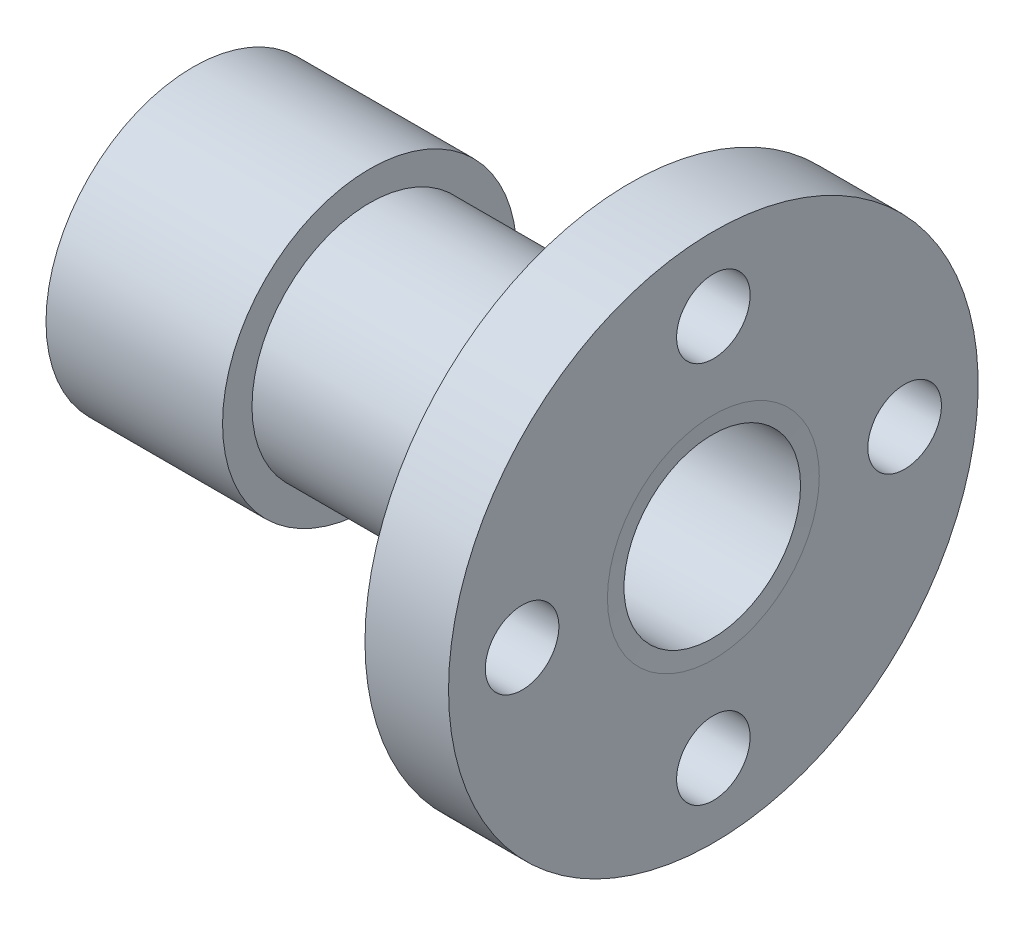
ISO-10303-21;
HEADER;
FILE_DESCRIPTION(('STEP AP214'),'2;1');
FILE_NAME('part.step','',(''),(''),'','','');
FILE_SCHEMA(('AUTOMOTIVE_DESIGN { 1 0 10303 214 1 1 1 1 }'));
ENDSEC;
DATA;
#1=APPLICATION_CONTEXT('core data for automotive mechanical design processes');
#2=APPLICATION_PROTOCOL_DEFINITION('international standard','automotive_design',2000,#1);
#3=PRODUCT_CONTEXT('',#1,'mechanical');
#4=PRODUCT('Part','Part','',(#3));
#5=PRODUCT_RELATED_PRODUCT_CATEGORY('part','',(#4));
#6=PRODUCT_DEFINITION_FORMATION('','',#4);
#7=PRODUCT_DEFINITION_CONTEXT('part definition',#1,'design');
#8=PRODUCT_DEFINITION('design','',#6,#7);
#9=PRODUCT_DEFINITION_SHAPE('','',#8);
#10=(LENGTH_UNIT() NAMED_UNIT(*) SI_UNIT(.MILLI.,.METRE.));
#11=(NAMED_UNIT(*) PLANE_ANGLE_UNIT() SI_UNIT($,.RADIAN.));
#12=(NAMED_UNIT(*) SI_UNIT($,.STERADIAN.) SOLID_ANGLE_UNIT());
#13=UNCERTAINTY_MEASURE_WITH_UNIT(LENGTH_MEASURE(1.E-05),#10,'distance_accuracy_value','');
#14=(GEOMETRIC_REPRESENTATION_CONTEXT(3) GLOBAL_UNCERTAINTY_ASSIGNED_CONTEXT((#13)) GLOBAL_UNIT_ASSIGNED_CONTEXT((#10,
#11,#12)) REPRESENTATION_CONTEXT('',''));
#15=CARTESIAN_POINT('',(0.,0.,0.));
#16=DIRECTION('',(0.,0.,1.));
#17=DIRECTION('',(1.,0.,0.));
#18=AXIS2_PLACEMENT_3D('',#15,#16,#17);
#19=CARTESIAN_POINT('',(0.,0.,0.));
#20=DIRECTION('',(-1.,0.,0.));
#21=DIRECTION('',(0.,0.,1.));
#22=AXIS2_PLACEMENT_3D('',#19,#20,#21);
#23=PLANE('',#22);
#24=CARTESIAN_POINT('',(0.,0.,0.));
#25=DIRECTION('',(-1.,0.,0.));
#26=DIRECTION('',(0.,0.,1.));
#27=AXIS2_PLACEMENT_3D('',#24,#25,#26);
#28=CIRCLE('',#27,18.0000000000002);
#29=CARTESIAN_POINT('',(0.,0.,-18.0000000000002));
#30=VERTEX_POINT('',#29);
#31=EDGE_CURVE('E10',#30,#30,#28,.T.);
#32=ORIENTED_EDGE('',*,*,#31,.T.);
#33=EDGE_LOOP('',(#32));
#34=FACE_BOUND('',#33,.T.);
#35=CARTESIAN_POINT('',(0.,-32.5,0.));
#36=DIRECTION('',(-1.,0.,0.));
#37=DIRECTION('',(0.,0.,1.));
#38=AXIS2_PLACEMENT_3D('',#35,#36,#37);
#39=CIRCLE('',#38,6.25);
#40=CARTESIAN_POINT('',(0.,-32.5,6.25));
#41=VERTEX_POINT('',#40);
#42=EDGE_CURVE('E75',#41,#41,#39,.T.);
#43=ORIENTED_EDGE('',*,*,#42,.T.);
#44=EDGE_LOOP('',(#43));
#45=FACE_BOUND('',#44,.T.);
#46=CARTESIAN_POINT('',(0.,0.,-32.5));
#47=DIRECTION('',(-1.,0.,0.));
#48=DIRECTION('',(0.,0.,1.));
#49=AXIS2_PLACEMENT_3D('',#46,#47,#48);
#50=CIRCLE('',#49,6.24999999999989);
#51=CARTESIAN_POINT('',(0.,0.,-26.2500000000001));
#52=VERTEX_POINT('',#51);
#53=EDGE_CURVE('E90',#52,#52,#50,.T.);
#54=ORIENTED_EDGE('',*,*,#53,.T.);
#55=EDGE_LOOP('',(#54));
#56=FACE_BOUND('',#55,.T.);
#57=CARTESIAN_POINT('',(0.,32.5,2.26946287024804E-13));
#58=DIRECTION('',(-1.,0.,0.));
#59=DIRECTION('',(0.,0.,1.));
#60=AXIS2_PLACEMENT_3D('',#57,#58,#59);
#61=CIRCLE('',#60,6.25);
#62=CARTESIAN_POINT('',(0.,32.5,6.25000000000023));
#63=VERTEX_POINT('',#62);
#64=EDGE_CURVE('E83',#63,#63,#61,.T.);
#65=ORIENTED_EDGE('',*,*,#64,.T.);
#66=EDGE_LOOP('',(#65));
#67=FACE_BOUND('',#66,.T.);
#68=CARTESIAN_POINT('',(0.,-3.40419430537206E-13,32.5));
#69=DIRECTION('',(-1.,0.,0.));
#70=DIRECTION('',(0.,0.,1.));
#71=AXIS2_PLACEMENT_3D('',#68,#69,#70);
#72=CIRCLE('',#71,6.25);
#73=CARTESIAN_POINT('',(0.,-3.40419430537206E-13,38.75));
#74=VERTEX_POINT('',#73);
#75=EDGE_CURVE('E76',#74,#74,#72,.T.);
#76=ORIENTED_EDGE('',*,*,#75,.T.);
#77=EDGE_LOOP('',(#76));
#78=FACE_BOUND('',#77,.T.);
#79=CARTESIAN_POINT('',(0.,0.,0.));
#80=DIRECTION('',(-1.,0.,0.));
#81=DIRECTION('',(0.,0.,1.));
#82=AXIS2_PLACEMENT_3D('',#79,#80,#81);
#83=CIRCLE('',#82,45.);
#84=CARTESIAN_POINT('',(0.,0.,45.));
#85=VERTEX_POINT('',#84);
#86=EDGE_CURVE('E51',#85,#85,#83,.T.);
#87=ORIENTED_EDGE('',*,*,#86,.F.);
#88=EDGE_LOOP('',(#87));
#89=FACE_BOUND('',#88,.T.);
#90=ADVANCED_FACE('F39',(#34,#45,#56,#67,#78,#89),#23,.F.);
#91=CARTESIAN_POINT('',(-88.4,0.,0.));
#92=DIRECTION('',(-1.,0.,0.));
#93=DIRECTION('',(0.,0.,1.));
#94=AXIS2_PLACEMENT_3D('',#91,#92,#93);
#95=CYLINDRICAL_SURFACE('',#94,45.);
#96=CARTESIAN_POINT('',(-14.2,0.,0.));
#97=DIRECTION('',(-1.,0.,0.));
#98=DIRECTION('',(0.,0.,1.));
#99=AXIS2_PLACEMENT_3D('',#96,#97,#98);
#100=CIRCLE('',#99,45.);
#101=CARTESIAN_POINT('',(-14.2,0.,45.));
#102=VERTEX_POINT('',#101);
#103=EDGE_CURVE('E54',#102,#102,#100,.T.);
#104=ORIENTED_EDGE('',*,*,#103,.F.);
#105=EDGE_LOOP('',(#104));
#106=FACE_BOUND('',#105,.T.);
#107=ORIENTED_EDGE('',*,*,#86,.T.);
#108=EDGE_LOOP('',(#107));
#109=FACE_BOUND('',#108,.T.);
#110=ADVANCED_FACE('F120',(#106,#109),#95,.T.);
#111=CARTESIAN_POINT('',(-14.2,45.,0.));
#112=DIRECTION('',(1.,0.,0.));
#113=DIRECTION('',(0.,0.,-1.));
#114=AXIS2_PLACEMENT_3D('',#111,#112,#113);
#115=PLANE('',#114);
#116=CARTESIAN_POINT('',(-14.2,-32.5,0.));
#117=DIRECTION('',(-1.,0.,0.));
#118=DIRECTION('',(0.,0.,1.));
#119=AXIS2_PLACEMENT_3D('',#116,#117,#118);
#120=CIRCLE('',#119,6.25);
#121=CARTESIAN_POINT('',(-14.2,-32.5,6.25));
#122=VERTEX_POINT('',#121);
#123=EDGE_CURVE('E95',#122,#122,#120,.T.);
#124=ORIENTED_EDGE('',*,*,#123,.F.);
#125=EDGE_LOOP('',(#124));
#126=FACE_BOUND('',#125,.T.);
#127=CARTESIAN_POINT('',(-14.2,0.,-32.5));
#128=DIRECTION('',(-1.,0.,0.));
#129=DIRECTION('',(0.,0.,1.));
#130=AXIS2_PLACEMENT_3D('',#127,#128,#129);
#131=CIRCLE('',#130,6.24999999999989);
#132=CARTESIAN_POINT('',(-14.2,0.,-26.2500000000001));
#133=VERTEX_POINT('',#132);
#134=EDGE_CURVE('E88',#133,#133,#131,.T.);
#135=ORIENTED_EDGE('',*,*,#134,.F.);
#136=EDGE_LOOP('',(#135));
#137=FACE_BOUND('',#136,.T.);
#138=CARTESIAN_POINT('',(-14.2,32.5,2.26946287024804E-13));
#139=DIRECTION('',(-1.,0.,0.));
#140=DIRECTION('',(0.,0.,1.));
#141=AXIS2_PLACEMENT_3D('',#138,#139,#140);
#142=CIRCLE('',#141,6.25);
#143=CARTESIAN_POINT('',(-14.2,32.5,6.25000000000023));
#144=VERTEX_POINT('',#143);
#145=EDGE_CURVE('E80',#144,#144,#142,.T.);
#146=ORIENTED_EDGE('',*,*,#145,.F.);
#147=EDGE_LOOP('',(#146));
#148=FACE_BOUND('',#147,.T.);
#149=CARTESIAN_POINT('',(-14.2,-3.40419430537206E-13,32.5));
#150=DIRECTION('',(-1.,0.,0.));
#151=DIRECTION('',(0.,0.,1.));
#152=AXIS2_PLACEMENT_3D('',#149,#150,#151);
#153=CIRCLE('',#152,6.25);
#154=CARTESIAN_POINT('',(-14.2,-3.40419430537206E-13,38.75));
#155=VERTEX_POINT('',#154);
#156=EDGE_CURVE('E71',#155,#155,#153,.T.);
#157=ORIENTED_EDGE('',*,*,#156,.F.);
#158=EDGE_LOOP('',(#157));
#159=FACE_BOUND('',#158,.T.);
#160=CARTESIAN_POINT('',(-14.2,0.,0.));
#161=DIRECTION('',(-1.,0.,0.));
#162=DIRECTION('',(0.,0.,1.));
#163=AXIS2_PLACEMENT_3D('',#160,#161,#162);
#164=CIRCLE('',#163,20.);
#165=CARTESIAN_POINT('',(-14.2,0.,20.));
#166=VERTEX_POINT('',#165);
#167=EDGE_CURVE('E58',#166,#166,#164,.T.);
#168=ORIENTED_EDGE('',*,*,#167,.F.);
#169=EDGE_LOOP('',(#168));
#170=FACE_BOUND('',#169,.T.);
#171=ORIENTED_EDGE('',*,*,#103,.T.);
#172=EDGE_LOOP('',(#171));
#173=FACE_BOUND('',#172,.T.);
#174=ADVANCED_FACE('F122',(#126,#137,#148,#159,#170,#173),#115,.F.);
#175=CARTESIAN_POINT('',(-88.4,0.,0.));
#176=DIRECTION('',(-1.,0.,0.));
#177=DIRECTION('',(0.,0.,1.));
#178=AXIS2_PLACEMENT_3D('',#175,#176,#177);
#179=CYLINDRICAL_SURFACE('',#178,20.);
#180=CARTESIAN_POINT('',(-58.4,0.,0.));
#181=DIRECTION('',(-1.,0.,0.));
#182=DIRECTION('',(0.,0.,1.));
#183=AXIS2_PLACEMENT_3D('',#180,#181,#182);
#184=CIRCLE('',#183,20.);
#185=CARTESIAN_POINT('',(-58.4,0.,20.));
#186=VERTEX_POINT('',#185);
#187=EDGE_CURVE('E64',#186,#186,#184,.T.);
#188=ORIENTED_EDGE('',*,*,#187,.F.);
#189=EDGE_LOOP('',(#188));
#190=FACE_BOUND('',#189,.T.);
#191=ORIENTED_EDGE('',*,*,#167,.T.);
#192=EDGE_LOOP('',(#191));
#193=FACE_BOUND('',#192,.T.);
#194=ADVANCED_FACE('F131',(#190,#193),#179,.T.);
#195=CARTESIAN_POINT('',(-58.4,20.,0.));
#196=DIRECTION('',(-1.,0.,0.));
#197=DIRECTION('',(0.,0.,1.));
#198=AXIS2_PLACEMENT_3D('',#195,#196,#197);
#199=PLANE('',#198);
#200=CARTESIAN_POINT('',(-58.4,0.,0.));
#201=DIRECTION('',(-1.,0.,0.));
#202=DIRECTION('',(0.,0.,1.));
#203=AXIS2_PLACEMENT_3D('',#200,#201,#202);
#204=CIRCLE('',#203,25.);
#205=CARTESIAN_POINT('',(-58.4,0.,25.));
#206=VERTEX_POINT('',#205);
#207=EDGE_CURVE('E66',#206,#206,#204,.T.);
#208=ORIENTED_EDGE('',*,*,#207,.F.);
#209=EDGE_LOOP('',(#208));
#210=FACE_BOUND('',#209,.T.);
#211=ORIENTED_EDGE('',*,*,#187,.T.);
#212=EDGE_LOOP('',(#211));
#213=FACE_BOUND('',#212,.T.);
#214=ADVANCED_FACE('F135',(#210,#213),#199,.F.);
#215=CARTESIAN_POINT('',(-88.4,0.,0.));
#216=DIRECTION('',(-1.,0.,0.));
#217=DIRECTION('',(0.,0.,1.));
#218=AXIS2_PLACEMENT_3D('',#215,#216,#217);
#219=CYLINDRICAL_SURFACE('',#218,25.);
#220=CARTESIAN_POINT('',(-88.4,0.,0.));
#221=DIRECTION('',(-1.,0.,0.));
#222=DIRECTION('',(0.,0.,1.));
#223=AXIS2_PLACEMENT_3D('',#220,#221,#222);
#224=CIRCLE('',#223,25.);
#225=CARTESIAN_POINT('',(-88.4,0.,25.));
#226=VERTEX_POINT('',#225);
#227=EDGE_CURVE('E67',#226,#226,#224,.T.);
#228=ORIENTED_EDGE('',*,*,#227,.F.);
#229=EDGE_LOOP('',(#228));
#230=FACE_BOUND('',#229,.T.);
#231=ORIENTED_EDGE('',*,*,#207,.T.);
#232=EDGE_LOOP('',(#231));
#233=FACE_BOUND('',#232,.T.);
#234=ADVANCED_FACE('F137',(#230,#233),#219,.T.);
#235=CARTESIAN_POINT('',(-88.4,25.,0.));
#236=DIRECTION('',(1.,0.,0.));
#237=DIRECTION('',(0.,0.,-1.));
#238=AXIS2_PLACEMENT_3D('',#235,#236,#237);
#239=PLANE('',#238);
#240=CARTESIAN_POINT('',(-88.4,0.,0.));
#241=DIRECTION('',(-1.,0.,0.));
#242=DIRECTION('',(0.,0.,1.));
#243=AXIS2_PLACEMENT_3D('',#240,#241,#242);
#244=CIRCLE('',#243,19.);
#245=CARTESIAN_POINT('',(-88.4,0.,19.));
#246=VERTEX_POINT('',#245);
#247=EDGE_CURVE('E100',#246,#246,#244,.T.);
#248=ORIENTED_EDGE('',*,*,#247,.F.);
#249=EDGE_LOOP('',(#248));
#250=FACE_BOUND('',#249,.T.);
#251=ORIENTED_EDGE('',*,*,#227,.T.);
#252=EDGE_LOOP('',(#251));
#253=FACE_BOUND('',#252,.T.);
#254=ADVANCED_FACE('F141',(#250,#253),#239,.F.);
#255=CARTESIAN_POINT('',(0.,-3.40419430537206E-13,32.5));
#256=DIRECTION('',(-1.,0.,0.));
#257=DIRECTION('',(0.,0.,1.));
#258=AXIS2_PLACEMENT_3D('',#255,#256,#257);
#259=CYLINDRICAL_SURFACE('',#258,6.25);
#260=CARTESIAN_POINT('',(0.,-3.40419430537206E-13,38.75));
#261=CARTESIAN_POINT('',(-0.147916666666667,-3.40419430537206E-13,38.75));
#262=CARTESIAN_POINT('',(-0.295833333333333,-3.40419430537206E-13,38.75));
#263=CARTESIAN_POINT('',(-0.591666666666666,-3.40419430537206E-13,38.75));
#264=CARTESIAN_POINT('',(-0.739583333333333,-3.40419430537206E-13,38.75));
#265=CARTESIAN_POINT('',(-1.03541666666667,-3.40419430537206E-13,38.75));
#266=CARTESIAN_POINT('',(-1.18333333333333,-3.40419430537206E-13,38.75));
#267=CARTESIAN_POINT('',(-1.47916666666667,-3.40419430537206E-13,38.75));
#268=CARTESIAN_POINT('',(-1.62708333333333,-3.40419430537206E-13,38.75));
#269=CARTESIAN_POINT('',(-1.92291666666667,-3.40419430537206E-13,38.75));
#270=CARTESIAN_POINT('',(-2.07083333333333,-3.40419430537206E-13,38.75));
#271=CARTESIAN_POINT('',(-2.36666666666667,-3.40419430537206E-13,38.75));
#272=CARTESIAN_POINT('',(-2.51458333333333,-3.40419430537206E-13,38.75));
#273=CARTESIAN_POINT('',(-2.81041666666667,-3.40419430537206E-13,38.75));
#274=CARTESIAN_POINT('',(-2.95833333333333,-3.40419430537206E-13,38.75));
#275=CARTESIAN_POINT('',(-3.25416666666667,-3.40419430537206E-13,38.75));
#276=CARTESIAN_POINT('',(-3.40208333333333,-3.40419430537206E-13,38.75));
#277=CARTESIAN_POINT('',(-3.69791666666667,-3.40419430537206E-13,38.75));
#278=CARTESIAN_POINT('',(-3.84583333333333,-3.40419430537206E-13,38.75));
#279=CARTESIAN_POINT('',(-4.14166666666666,-3.40419430537206E-13,38.75));
#280=CARTESIAN_POINT('',(-4.28958333333333,-3.40419430537206E-13,38.75));
#281=CARTESIAN_POINT('',(-4.58541666666666,-3.40419430537206E-13,38.75));
#282=CARTESIAN_POINT('',(-4.73333333333333,-3.40419430537206E-13,38.75));
#283=CARTESIAN_POINT('',(-5.02916666666667,-3.40419430537206E-13,38.75));
#284=CARTESIAN_POINT('',(-5.17708333333333,-3.40419430537206E-13,38.75));
#285=CARTESIAN_POINT('',(-5.47291666666666,-3.40419430537206E-13,38.75));
#286=CARTESIAN_POINT('',(-5.62083333333333,-3.40419430537206E-13,38.75));
#287=CARTESIAN_POINT('',(-5.91666666666666,-3.40419430537206E-13,38.75));
#288=CARTESIAN_POINT('',(-6.06458333333333,-3.40419430537206E-13,38.75));
#289=CARTESIAN_POINT('',(-6.36041666666666,-3.40419430537206E-13,38.75));
#290=CARTESIAN_POINT('',(-6.50833333333333,-3.40419430537206E-13,38.75));
#291=CARTESIAN_POINT('',(-6.80416666666667,-3.40419430537206E-13,38.75));
#292=CARTESIAN_POINT('',(-6.95208333333333,-3.40419430537206E-13,38.75));
#293=CARTESIAN_POINT('',(-7.24791666666667,-3.40419430537206E-13,38.75));
#294=CARTESIAN_POINT('',(-7.39583333333333,-3.40419430537206E-13,38.75));
#295=CARTESIAN_POINT('',(-7.69166666666666,-3.40419430537206E-13,38.75));
#296=CARTESIAN_POINT('',(-7.83958333333333,-3.40419430537206E-13,38.75));
#297=CARTESIAN_POINT('',(-8.13541666666666,-3.40419430537206E-13,38.75));
#298=CARTESIAN_POINT('',(-8.28333333333333,-3.40419430537206E-13,38.75));
#299=CARTESIAN_POINT('',(-8.57916666666666,-3.40419430537206E-13,38.75));
#300=CARTESIAN_POINT('',(-8.72708333333333,-3.40419430537206E-13,38.75));
#301=CARTESIAN_POINT('',(-9.02291666666666,-3.40419430537206E-13,38.75));
#302=CARTESIAN_POINT('',(-9.17083333333333,-3.40419430537206E-13,38.75));
#303=CARTESIAN_POINT('',(-9.46666666666666,-3.40419430537206E-13,38.75));
#304=CARTESIAN_POINT('',(-9.61458333333333,-3.40419430537206E-13,38.75));
#305=CARTESIAN_POINT('',(-9.91041666666666,-3.40419430537206E-13,38.75));
#306=CARTESIAN_POINT('',(-10.0583333333333,-3.40419430537206E-13,38.75));
#307=CARTESIAN_POINT('',(-10.3541666666667,-3.40419430537206E-13,38.75));
#308=CARTESIAN_POINT('',(-10.5020833333333,-3.40419430537206E-13,38.75));
#309=CARTESIAN_POINT('',(-10.7979166666667,-3.40419430537206E-13,38.75));
#310=CARTESIAN_POINT('',(-10.9458333333333,-3.40419430537206E-13,38.75));
#311=CARTESIAN_POINT('',(-11.2416666666667,-3.40419430537206E-13,38.75));
#312=CARTESIAN_POINT('',(-11.3895833333333,-3.40419430537206E-13,38.75));
#313=CARTESIAN_POINT('',(-11.6854166666667,-3.40419430537206E-13,38.75));
#314=CARTESIAN_POINT('',(-11.8333333333333,-3.40419430537206E-13,38.75));
#315=CARTESIAN_POINT('',(-12.1291666666667,-3.40419430537206E-13,38.75));
#316=CARTESIAN_POINT('',(-12.2770833333333,-3.40419430537206E-13,38.75));
#317=CARTESIAN_POINT('',(-12.5729166666667,-3.40419430537206E-13,38.75));
#318=CARTESIAN_POINT('',(-12.7208333333333,-3.40419430537206E-13,38.75));
#319=CARTESIAN_POINT('',(-13.0166666666667,-3.40419430537206E-13,38.75));
#320=CARTESIAN_POINT('',(-13.1645833333333,-3.40419430537206E-13,38.75));
#321=CARTESIAN_POINT('',(-13.4604166666667,-3.40419430537206E-13,38.75));
#322=CARTESIAN_POINT('',(-13.6083333333333,-3.40419430537206E-13,38.75));
#323=CARTESIAN_POINT('',(-13.9041666666667,-3.40419430537206E-13,38.75));
#324=CARTESIAN_POINT('',(-14.0520833333333,-3.40419430537206E-13,38.75));
#325=CARTESIAN_POINT('',(-14.2,-3.40419430537206E-13,38.75));
#326=B_SPLINE_CURVE_WITH_KNOTS('',3,(#260,#261,#262,#263,#264,#265,#266,#267,#268,#269,#270,
#271,#272,#273,#274,#275,#276,#277,#278,#279,#280,#281,#282,#283,#284,#285,#286,#287,#288,#289,
#290,#291,#292,#293,#294,#295,#296,#297,#298,#299,#300,#301,#302,#303,#304,#305,#306,#307,#308,
#309,#310,#311,#312,#313,#314,#315,#316,#317,#318,#319,#320,#321,#322,#323,#324,#325),
.UNSPECIFIED.,.F.,.F.,(4,2,2,2,2,2,2,2,2,2,2,2,2,2,2,2,2,2,2,2,2,2,2,2,2,2,2,2,2,2,2,2,4),(0.,
0.44375,0.8875,1.33125,1.775,2.21875,2.6625,3.10625,3.55,3.99375,4.4375,4.88125,5.325,5.76875,
6.2125,6.65625,7.1,7.54375,7.9875,8.43125,8.875,9.31875,9.7625,10.20625,10.65,11.09375,11.5375,
11.98125,12.425,12.86875,13.3125,13.75625,14.2),.UNSPECIFIED.);
#327=EDGE_CURVE('BSEAM150',#74,#155,#326,.T.);
#328=ORIENTED_EDGE('',*,*,#75,.F.);
#329=ORIENTED_EDGE('',*,*,#156,.T.);
#330=ORIENTED_EDGE('',*,*,#327,.T.);
#331=ORIENTED_EDGE('',*,*,#327,.F.);
#332=EDGE_LOOP('',(#328,#330,#329,#331));
#333=FACE_BOUND('',#332,.T.);
#334=ADVANCED_FACE('F150',(#333),#259,.F.);
#335=CARTESIAN_POINT('',(0.,32.5,2.26946287024804E-13));
#336=DIRECTION('',(-1.,0.,0.));
#337=DIRECTION('',(0.,0.,1.));
#338=AXIS2_PLACEMENT_3D('',#335,#336,#337);
#339=CYLINDRICAL_SURFACE('',#338,6.25);
#340=CARTESIAN_POINT('',(0.,32.5,6.25000000000023));
#341=CARTESIAN_POINT('',(-0.147916666666667,32.5,6.25000000000023));
#342=CARTESIAN_POINT('',(-0.295833333333333,32.5,6.25000000000023));
#343=CARTESIAN_POINT('',(-0.591666666666666,32.5,6.25000000000023));
#344=CARTESIAN_POINT('',(-0.739583333333333,32.5,6.25000000000023));
#345=CARTESIAN_POINT('',(-1.03541666666667,32.5,6.25000000000023));
#346=CARTESIAN_POINT('',(-1.18333333333333,32.5,6.25000000000023));
#347=CARTESIAN_POINT('',(-1.47916666666667,32.5,6.25000000000023));
#348=CARTESIAN_POINT('',(-1.62708333333333,32.5,6.25000000000023));
#349=CARTESIAN_POINT('',(-1.92291666666667,32.5,6.25000000000023));
#350=CARTESIAN_POINT('',(-2.07083333333333,32.5,6.25000000000023));
#351=CARTESIAN_POINT('',(-2.36666666666667,32.5,6.25000000000023));
#352=CARTESIAN_POINT('',(-2.51458333333333,32.5,6.25000000000023));
#353=CARTESIAN_POINT('',(-2.81041666666667,32.5,6.25000000000023));
#354=CARTESIAN_POINT('',(-2.95833333333333,32.5,6.25000000000023));
#355=CARTESIAN_POINT('',(-3.25416666666667,32.5,6.25000000000023));
#356=CARTESIAN_POINT('',(-3.40208333333333,32.5,6.25000000000023));
#357=CARTESIAN_POINT('',(-3.69791666666667,32.5,6.25000000000023));
#358=CARTESIAN_POINT('',(-3.84583333333333,32.5,6.25000000000023));
#359=CARTESIAN_POINT('',(-4.14166666666666,32.5,6.25000000000023));
#360=CARTESIAN_POINT('',(-4.28958333333333,32.5,6.25000000000023));
#361=CARTESIAN_POINT('',(-4.58541666666666,32.5,6.25000000000023));
#362=CARTESIAN_POINT('',(-4.73333333333333,32.5,6.25000000000023));
#363=CARTESIAN_POINT('',(-5.02916666666667,32.5,6.25000000000023));
#364=CARTESIAN_POINT('',(-5.17708333333333,32.5,6.25000000000023));
#365=CARTESIAN_POINT('',(-5.47291666666666,32.5,6.25000000000023));
#366=CARTESIAN_POINT('',(-5.62083333333333,32.5,6.25000000000023));
#367=CARTESIAN_POINT('',(-5.91666666666666,32.5,6.25000000000023));
#368=CARTESIAN_POINT('',(-6.06458333333333,32.5,6.25000000000023));
#369=CARTESIAN_POINT('',(-6.36041666666666,32.5,6.25000000000023));
#370=CARTESIAN_POINT('',(-6.50833333333333,32.5,6.25000000000023));
#371=CARTESIAN_POINT('',(-6.80416666666667,32.5,6.25000000000023));
#372=CARTESIAN_POINT('',(-6.95208333333333,32.5,6.25000000000023));
#373=CARTESIAN_POINT('',(-7.24791666666667,32.5,6.25000000000023));
#374=CARTESIAN_POINT('',(-7.39583333333333,32.5,6.25000000000023));
#375=CARTESIAN_POINT('',(-7.69166666666666,32.5,6.25000000000023));
#376=CARTESIAN_POINT('',(-7.83958333333333,32.5,6.25000000000023));
#377=CARTESIAN_POINT('',(-8.13541666666666,32.5,6.25000000000023));
#378=CARTESIAN_POINT('',(-8.28333333333333,32.5,6.25000000000023));
#379=CARTESIAN_POINT('',(-8.57916666666666,32.5,6.25000000000023));
#380=CARTESIAN_POINT('',(-8.72708333333333,32.5,6.25000000000023));
#381=CARTESIAN_POINT('',(-9.02291666666666,32.5,6.25000000000023));
#382=CARTESIAN_POINT('',(-9.17083333333333,32.5,6.25000000000023));
#383=CARTESIAN_POINT('',(-9.46666666666666,32.5,6.25000000000023));
#384=CARTESIAN_POINT('',(-9.61458333333333,32.5,6.25000000000023));
#385=CARTESIAN_POINT('',(-9.91041666666666,32.5,6.25000000000023));
#386=CARTESIAN_POINT('',(-10.0583333333333,32.5,6.25000000000023));
#387=CARTESIAN_POINT('',(-10.3541666666667,32.5,6.25000000000023));
#388=CARTESIAN_POINT('',(-10.5020833333333,32.5,6.25000000000023));
#389=CARTESIAN_POINT('',(-10.7979166666667,32.5,6.25000000000023));
#390=CARTESIAN_POINT('',(-10.9458333333333,32.5,6.25000000000023));
#391=CARTESIAN_POINT('',(-11.2416666666667,32.5,6.25000000000023));
#392=CARTESIAN_POINT('',(-11.3895833333333,32.5,6.25000000000023));
#393=CARTESIAN_POINT('',(-11.6854166666667,32.5,6.25000000000023));
#394=CARTESIAN_POINT('',(-11.8333333333333,32.5,6.25000000000023));
#395=CARTESIAN_POINT('',(-12.1291666666667,32.5,6.25000000000023));
#396=CARTESIAN_POINT('',(-12.2770833333333,32.5,6.25000000000023));
#397=CARTESIAN_POINT('',(-12.5729166666667,32.5,6.25000000000023));
#398=CARTESIAN_POINT('',(-12.7208333333333,32.5,6.25000000000023));
#399=CARTESIAN_POINT('',(-13.0166666666667,32.5,6.25000000000023));
#400=CARTESIAN_POINT('',(-13.1645833333333,32.5,6.25000000000023));
#401=CARTESIAN_POINT('',(-13.4604166666667,32.5,6.25000000000023));
#402=CARTESIAN_POINT('',(-13.6083333333333,32.5,6.25000000000023));
#403=CARTESIAN_POINT('',(-13.9041666666667,32.5,6.25000000000023));
#404=CARTESIAN_POINT('',(-14.0520833333333,32.5,6.25000000000023));
#405=CARTESIAN_POINT('',(-14.2,32.5,6.25000000000023));
#406=B_SPLINE_CURVE_WITH_KNOTS('',3,(#340,#341,#342,#343,#344,#345,#346,#347,#348,#349,#350,
#351,#352,#353,#354,#355,#356,#357,#358,#359,#360,#361,#362,#363,#364,#365,#366,#367,#368,#369,
#370,#371,#372,#373,#374,#375,#376,#377,#378,#379,#380,#381,#382,#383,#384,#385,#386,#387,#388,
#389,#390,#391,#392,#393,#394,#395,#396,#397,#398,#399,#400,#401,#402,#403,#404,#405),
.UNSPECIFIED.,.F.,.F.,(4,2,2,2,2,2,2,2,2,2,2,2,2,2,2,2,2,2,2,2,2,2,2,2,2,2,2,2,2,2,2,2,4),(0.,
0.44375,0.8875,1.33125,1.775,2.21875,2.6625,3.10625,3.55,3.99375,4.4375,4.88125,5.325,5.76875,
6.2125,6.65625,7.1,7.54375,7.9875,8.43125,8.875,9.31875,9.7625,10.20625,10.65,11.09375,11.5375,
11.98125,12.425,12.86875,13.3125,13.75625,14.2),.UNSPECIFIED.);
#407=EDGE_CURVE('BSEAM151',#63,#144,#406,.T.);
#408=ORIENTED_EDGE('',*,*,#64,.F.);
#409=ORIENTED_EDGE('',*,*,#145,.T.);
#410=ORIENTED_EDGE('',*,*,#407,.T.);
#411=ORIENTED_EDGE('',*,*,#407,.F.);
#412=EDGE_LOOP('',(#408,#410,#409,#411));
#413=FACE_BOUND('',#412,.T.);
#414=ADVANCED_FACE('F151',(#413),#339,.F.);
#415=CARTESIAN_POINT('',(0.,0.,-32.5));
#416=DIRECTION('',(-1.,0.,0.));
#417=DIRECTION('',(0.,0.,1.));
#418=AXIS2_PLACEMENT_3D('',#415,#416,#417);
#419=CYLINDRICAL_SURFACE('',#418,6.24999999999989);
#420=CARTESIAN_POINT('',(0.,0.,-26.2500000000001));
#421=CARTESIAN_POINT('',(-0.147916666666667,0.,-26.2500000000001));
#422=CARTESIAN_POINT('',(-0.295833333333333,0.,-26.2500000000001));
#423=CARTESIAN_POINT('',(-0.591666666666666,0.,-26.2500000000001));
#424=CARTESIAN_POINT('',(-0.739583333333333,0.,-26.2500000000001));
#425=CARTESIAN_POINT('',(-1.03541666666667,0.,-26.2500000000001));
#426=CARTESIAN_POINT('',(-1.18333333333333,0.,-26.2500000000001));
#427=CARTESIAN_POINT('',(-1.47916666666667,0.,-26.2500000000001));
#428=CARTESIAN_POINT('',(-1.62708333333333,0.,-26.2500000000001));
#429=CARTESIAN_POINT('',(-1.92291666666667,0.,-26.2500000000001));
#430=CARTESIAN_POINT('',(-2.07083333333333,0.,-26.2500000000001));
#431=CARTESIAN_POINT('',(-2.36666666666667,0.,-26.2500000000001));
#432=CARTESIAN_POINT('',(-2.51458333333333,0.,-26.2500000000001));
#433=CARTESIAN_POINT('',(-2.81041666666667,0.,-26.2500000000001));
#434=CARTESIAN_POINT('',(-2.95833333333333,0.,-26.2500000000001));
#435=CARTESIAN_POINT('',(-3.25416666666667,0.,-26.2500000000001));
#436=CARTESIAN_POINT('',(-3.40208333333333,0.,-26.2500000000001));
#437=CARTESIAN_POINT('',(-3.69791666666667,0.,-26.2500000000001));
#438=CARTESIAN_POINT('',(-3.84583333333333,0.,-26.2500000000001));
#439=CARTESIAN_POINT('',(-4.14166666666666,0.,-26.2500000000001));
#440=CARTESIAN_POINT('',(-4.28958333333333,0.,-26.2500000000001));
#441=CARTESIAN_POINT('',(-4.58541666666666,0.,-26.2500000000001));
#442=CARTESIAN_POINT('',(-4.73333333333333,0.,-26.2500000000001));
#443=CARTESIAN_POINT('',(-5.02916666666667,0.,-26.2500000000001));
#444=CARTESIAN_POINT('',(-5.17708333333333,0.,-26.2500000000001));
#445=CARTESIAN_POINT('',(-5.47291666666666,0.,-26.2500000000001));
#446=CARTESIAN_POINT('',(-5.62083333333333,0.,-26.2500000000001));
#447=CARTESIAN_POINT('',(-5.91666666666666,0.,-26.2500000000001));
#448=CARTESIAN_POINT('',(-6.06458333333333,0.,-26.2500000000001));
#449=CARTESIAN_POINT('',(-6.36041666666666,0.,-26.2500000000001));
#450=CARTESIAN_POINT('',(-6.50833333333333,0.,-26.2500000000001));
#451=CARTESIAN_POINT('',(-6.80416666666667,0.,-26.2500000000001));
#452=CARTESIAN_POINT('',(-6.95208333333333,0.,-26.2500000000001));
#453=CARTESIAN_POINT('',(-7.24791666666667,0.,-26.2500000000001));
#454=CARTESIAN_POINT('',(-7.39583333333333,0.,-26.2500000000001));
#455=CARTESIAN_POINT('',(-7.69166666666666,0.,-26.2500000000001));
#456=CARTESIAN_POINT('',(-7.83958333333333,0.,-26.2500000000001));
#457=CARTESIAN_POINT('',(-8.13541666666666,0.,-26.2500000000001));
#458=CARTESIAN_POINT('',(-8.28333333333333,0.,-26.2500000000001));
#459=CARTESIAN_POINT('',(-8.57916666666666,0.,-26.2500000000001));
#460=CARTESIAN_POINT('',(-8.72708333333333,0.,-26.2500000000001));
#461=CARTESIAN_POINT('',(-9.02291666666666,0.,-26.2500000000001));
#462=CARTESIAN_POINT('',(-9.17083333333333,0.,-26.2500000000001));
#463=CARTESIAN_POINT('',(-9.46666666666666,0.,-26.2500000000001));
#464=CARTESIAN_POINT('',(-9.61458333333333,0.,-26.2500000000001));
#465=CARTESIAN_POINT('',(-9.91041666666666,0.,-26.2500000000001));
#466=CARTESIAN_POINT('',(-10.0583333333333,0.,-26.2500000000001));
#467=CARTESIAN_POINT('',(-10.3541666666667,0.,-26.2500000000001));
#468=CARTESIAN_POINT('',(-10.5020833333333,0.,-26.2500000000001));
#469=CARTESIAN_POINT('',(-10.7979166666667,0.,-26.2500000000001));
#470=CARTESIAN_POINT('',(-10.9458333333333,0.,-26.2500000000001));
#471=CARTESIAN_POINT('',(-11.2416666666667,0.,-26.2500000000001));
#472=CARTESIAN_POINT('',(-11.3895833333333,0.,-26.2500000000001));
#473=CARTESIAN_POINT('',(-11.6854166666667,0.,-26.2500000000001));
#474=CARTESIAN_POINT('',(-11.8333333333333,0.,-26.2500000000001));
#475=CARTESIAN_POINT('',(-12.1291666666667,0.,-26.2500000000001));
#476=CARTESIAN_POINT('',(-12.2770833333333,0.,-26.2500000000001));
#477=CARTESIAN_POINT('',(-12.5729166666667,0.,-26.2500000000001));
#478=CARTESIAN_POINT('',(-12.7208333333333,0.,-26.2500000000001));
#479=CARTESIAN_POINT('',(-13.0166666666667,0.,-26.2500000000001));
#480=CARTESIAN_POINT('',(-13.1645833333333,0.,-26.2500000000001));
#481=CARTESIAN_POINT('',(-13.4604166666667,0.,-26.2500000000001));
#482=CARTESIAN_POINT('',(-13.6083333333333,0.,-26.2500000000001));
#483=CARTESIAN_POINT('',(-13.9041666666667,0.,-26.2500000000001));
#484=CARTESIAN_POINT('',(-14.0520833333333,0.,-26.2500000000001));
#485=CARTESIAN_POINT('',(-14.2,0.,-26.2500000000001));
#486=B_SPLINE_CURVE_WITH_KNOTS('',3,(#420,#421,#422,#423,#424,#425,#426,#427,#428,#429,#430,
#431,#432,#433,#434,#435,#436,#437,#438,#439,#440,#441,#442,#443,#444,#445,#446,#447,#448,#449,
#450,#451,#452,#453,#454,#455,#456,#457,#458,#459,#460,#461,#462,#463,#464,#465,#466,#467,#468,
#469,#470,#471,#472,#473,#474,#475,#476,#477,#478,#479,#480,#481,#482,#483,#484,#485),
.UNSPECIFIED.,.F.,.F.,(4,2,2,2,2,2,2,2,2,2,2,2,2,2,2,2,2,2,2,2,2,2,2,2,2,2,2,2,2,2,2,2,4),(0.,
0.44375,0.8875,1.33125,1.775,2.21875,2.6625,3.10625,3.55,3.99375,4.4375,4.88125,5.325,5.76875,
6.2125,6.65625,7.1,7.54375,7.9875,8.43125,8.875,9.31875,9.7625,10.20625,10.65,11.09375,11.5375,
11.98125,12.425,12.86875,13.3125,13.75625,14.2),.UNSPECIFIED.);
#487=EDGE_CURVE('BSEAM154',#52,#133,#486,.T.);
#488=ORIENTED_EDGE('',*,*,#53,.F.);
#489=ORIENTED_EDGE('',*,*,#134,.T.);
#490=ORIENTED_EDGE('',*,*,#487,.T.);
#491=ORIENTED_EDGE('',*,*,#487,.F.);
#492=EDGE_LOOP('',(#488,#490,#489,#491));
#493=FACE_BOUND('',#492,.T.);
#494=ADVANCED_FACE('F154',(#493),#419,.F.);
#495=CARTESIAN_POINT('',(0.,-32.5,0.));
#496=DIRECTION('',(-1.,0.,0.));
#497=DIRECTION('',(0.,0.,1.));
#498=AXIS2_PLACEMENT_3D('',#495,#496,#497);
#499=CYLINDRICAL_SURFACE('',#498,6.25);
#500=CARTESIAN_POINT('',(0.,-32.5,6.25));
#501=CARTESIAN_POINT('',(-0.147916666666667,-32.5,6.25));
#502=CARTESIAN_POINT('',(-0.295833333333333,-32.5,6.25));
#503=CARTESIAN_POINT('',(-0.591666666666666,-32.5,6.25));
#504=CARTESIAN_POINT('',(-0.739583333333333,-32.5,6.25));
#505=CARTESIAN_POINT('',(-1.03541666666667,-32.5,6.25));
#506=CARTESIAN_POINT('',(-1.18333333333333,-32.5,6.25));
#507=CARTESIAN_POINT('',(-1.47916666666667,-32.5,6.25));
#508=CARTESIAN_POINT('',(-1.62708333333333,-32.5,6.25));
#509=CARTESIAN_POINT('',(-1.92291666666667,-32.5,6.25));
#510=CARTESIAN_POINT('',(-2.07083333333333,-32.5,6.25));
#511=CARTESIAN_POINT('',(-2.36666666666667,-32.5,6.25));
#512=CARTESIAN_POINT('',(-2.51458333333333,-32.5,6.25));
#513=CARTESIAN_POINT('',(-2.81041666666667,-32.5,6.25));
#514=CARTESIAN_POINT('',(-2.95833333333333,-32.5,6.25));
#515=CARTESIAN_POINT('',(-3.25416666666667,-32.5,6.25));
#516=CARTESIAN_POINT('',(-3.40208333333333,-32.5,6.25));
#517=CARTESIAN_POINT('',(-3.69791666666667,-32.5,6.25));
#518=CARTESIAN_POINT('',(-3.84583333333333,-32.5,6.25));
#519=CARTESIAN_POINT('',(-4.14166666666666,-32.5,6.25));
#520=CARTESIAN_POINT('',(-4.28958333333333,-32.5,6.25));
#521=CARTESIAN_POINT('',(-4.58541666666666,-32.5,6.25));
#522=CARTESIAN_POINT('',(-4.73333333333333,-32.5,6.25));
#523=CARTESIAN_POINT('',(-5.02916666666667,-32.5,6.25));
#524=CARTESIAN_POINT('',(-5.17708333333333,-32.5,6.25));
#525=CARTESIAN_POINT('',(-5.47291666666666,-32.5,6.25));
#526=CARTESIAN_POINT('',(-5.62083333333333,-32.5,6.25));
#527=CARTESIAN_POINT('',(-5.91666666666666,-32.5,6.25));
#528=CARTESIAN_POINT('',(-6.06458333333333,-32.5,6.25));
#529=CARTESIAN_POINT('',(-6.36041666666666,-32.5,6.25));
#530=CARTESIAN_POINT('',(-6.50833333333333,-32.5,6.25));
#531=CARTESIAN_POINT('',(-6.80416666666667,-32.5,6.25));
#532=CARTESIAN_POINT('',(-6.95208333333333,-32.5,6.25));
#533=CARTESIAN_POINT('',(-7.24791666666667,-32.5,6.25));
#534=CARTESIAN_POINT('',(-7.39583333333333,-32.5,6.25));
#535=CARTESIAN_POINT('',(-7.69166666666666,-32.5,6.25));
#536=CARTESIAN_POINT('',(-7.83958333333333,-32.5,6.25));
#537=CARTESIAN_POINT('',(-8.13541666666666,-32.5,6.25));
#538=CARTESIAN_POINT('',(-8.28333333333333,-32.5,6.25));
#539=CARTESIAN_POINT('',(-8.57916666666666,-32.5,6.25));
#540=CARTESIAN_POINT('',(-8.72708333333333,-32.5,6.25));
#541=CARTESIAN_POINT('',(-9.02291666666666,-32.5,6.25));
#542=CARTESIAN_POINT('',(-9.17083333333333,-32.5,6.25));
#543=CARTESIAN_POINT('',(-9.46666666666666,-32.5,6.25));
#544=CARTESIAN_POINT('',(-9.61458333333333,-32.5,6.25));
#545=CARTESIAN_POINT('',(-9.91041666666666,-32.5,6.25));
#546=CARTESIAN_POINT('',(-10.0583333333333,-32.5,6.25));
#547=CARTESIAN_POINT('',(-10.3541666666667,-32.5,6.25));
#548=CARTESIAN_POINT('',(-10.5020833333333,-32.5,6.25));
#549=CARTESIAN_POINT('',(-10.7979166666667,-32.5,6.25));
#550=CARTESIAN_POINT('',(-10.9458333333333,-32.5,6.25));
#551=CARTESIAN_POINT('',(-11.2416666666667,-32.5,6.25));
#552=CARTESIAN_POINT('',(-11.3895833333333,-32.5,6.25));
#553=CARTESIAN_POINT('',(-11.6854166666667,-32.5,6.25));
#554=CARTESIAN_POINT('',(-11.8333333333333,-32.5,6.25));
#555=CARTESIAN_POINT('',(-12.1291666666667,-32.5,6.25));
#556=CARTESIAN_POINT('',(-12.2770833333333,-32.5,6.25));
#557=CARTESIAN_POINT('',(-12.5729166666667,-32.5,6.25));
#558=CARTESIAN_POINT('',(-12.7208333333333,-32.5,6.25));
#559=CARTESIAN_POINT('',(-13.0166666666667,-32.5,6.25));
#560=CARTESIAN_POINT('',(-13.1645833333333,-32.5,6.25));
#561=CARTESIAN_POINT('',(-13.4604166666667,-32.5,6.25));
#562=CARTESIAN_POINT('',(-13.6083333333333,-32.5,6.25));
#563=CARTESIAN_POINT('',(-13.9041666666667,-32.5,6.25));
#564=CARTESIAN_POINT('',(-14.0520833333333,-32.5,6.25));
#565=CARTESIAN_POINT('',(-14.2,-32.5,6.25));
#566=B_SPLINE_CURVE_WITH_KNOTS('',3,(#500,#501,#502,#503,#504,#505,#506,#507,#508,#509,#510,
#511,#512,#513,#514,#515,#516,#517,#518,#519,#520,#521,#522,#523,#524,#525,#526,#527,#528,#529,
#530,#531,#532,#533,#534,#535,#536,#537,#538,#539,#540,#541,#542,#543,#544,#545,#546,#547,#548,
#549,#550,#551,#552,#553,#554,#555,#556,#557,#558,#559,#560,#561,#562,#563,#564,#565),
.UNSPECIFIED.,.F.,.F.,(4,2,2,2,2,2,2,2,2,2,2,2,2,2,2,2,2,2,2,2,2,2,2,2,2,2,2,2,2,2,2,2,4),(0.,
0.44375,0.8875,1.33125,1.775,2.21875,2.6625,3.10625,3.55,3.99375,4.4375,4.88125,5.325,5.76875,
6.2125,6.65625,7.1,7.54375,7.9875,8.43125,8.875,9.31875,9.7625,10.20625,10.65,11.09375,11.5375,
11.98125,12.425,12.86875,13.3125,13.75625,14.2),.UNSPECIFIED.);
#567=EDGE_CURVE('BSEAM157',#41,#122,#566,.T.);
#568=ORIENTED_EDGE('',*,*,#42,.F.);
#569=ORIENTED_EDGE('',*,*,#123,.T.);
#570=ORIENTED_EDGE('',*,*,#567,.T.);
#571=ORIENTED_EDGE('',*,*,#567,.F.);
#572=EDGE_LOOP('',(#568,#570,#569,#571));
#573=FACE_BOUND('',#572,.T.);
#574=ADVANCED_FACE('F157',(#573),#499,.F.);
#575=CARTESIAN_POINT('',(-64.4,0.,0.));
#576=DIRECTION('',(-1.,0.,0.));
#577=DIRECTION('',(0.,0.,1.));
#578=AXIS2_PLACEMENT_3D('',#575,#576,#577);
#579=CYLINDRICAL_SURFACE('',#578,19.);
#580=CARTESIAN_POINT('',(-64.4,0.,0.));
#581=DIRECTION('',(-1.,0.,0.));
#582=DIRECTION('',(0.,0.,1.));
#583=AXIS2_PLACEMENT_3D('',#580,#581,#582);
#584=CIRCLE('',#583,19.);
#585=CARTESIAN_POINT('',(-64.4,0.,19.));
#586=VERTEX_POINT('',#585);
#587=EDGE_CURVE('E77',#586,#586,#584,.T.);
#588=ORIENTED_EDGE('',*,*,#587,.F.);
#589=EDGE_LOOP('',(#588));
#590=FACE_BOUND('',#589,.T.);
#591=ORIENTED_EDGE('',*,*,#247,.T.);
#592=EDGE_LOOP('',(#591));
#593=FACE_BOUND('',#592,.T.);
#594=ADVANCED_FACE('F119',(#590,#593),#579,.F.);
#595=CARTESIAN_POINT('',(-64.4,0.,0.));
#596=DIRECTION('',(-1.,0.,0.));
#597=DIRECTION('',(0.,0.,1.));
#598=AXIS2_PLACEMENT_3D('',#595,#596,#597);
#599=PLANE('',#598);
#600=CARTESIAN_POINT('',(-64.4,0.,0.));
#601=DIRECTION('',(-1.,0.,0.));
#602=DIRECTION('',(0.,0.,1.));
#603=AXIS2_PLACEMENT_3D('',#600,#601,#602);
#604=CIRCLE('',#603,15.);
#605=CARTESIAN_POINT('',(-64.4,0.,15.));
#606=VERTEX_POINT('',#605);
#607=EDGE_CURVE('E99',#606,#606,#604,.F.);
#608=ORIENTED_EDGE('',*,*,#607,.T.);
#609=EDGE_LOOP('',(#608));
#610=FACE_BOUND('',#609,.T.);
#611=ORIENTED_EDGE('',*,*,#587,.T.);
#612=EDGE_LOOP('',(#611));
#613=FACE_BOUND('',#612,.T.);
#614=ADVANCED_FACE('F106',(#610,#613),#599,.T.);
#615=CARTESIAN_POINT('',(-88.401,0.,0.));
#616=DIRECTION('',(1.,0.,0.));
#617=DIRECTION('',(0.,0.,-1.));
#618=AXIS2_PLACEMENT_3D('',#615,#616,#617);
#619=CYLINDRICAL_SURFACE('',#618,15.);
#620=CARTESIAN_POINT('',(-0.183487860451456,0.,0.));
#621=DIRECTION('',(-1.,0.,0.));
#622=DIRECTION('',(0.,0.,1.));
#623=AXIS2_PLACEMENT_3D('',#620,#621,#622);
#624=CIRCLE('',#623,15.);
#625=CARTESIAN_POINT('',(-0.183487860451456,0.,-15.));
#626=VERTEX_POINT('',#625);
#627=EDGE_CURVE('E50',#626,#626,#624,.F.);
#628=ORIENTED_EDGE('',*,*,#627,.T.);
#629=EDGE_LOOP('',(#628));
#630=FACE_BOUND('',#629,.T.);
#631=ORIENTED_EDGE('',*,*,#607,.F.);
#632=EDGE_LOOP('',(#631));
#633=FACE_BOUND('',#632,.T.);
#634=ADVANCED_FACE('F108',(#630,#633),#619,.F.);
#635=CARTESIAN_POINT('',(-0.183487860451456,0.,0.));
#636=DIRECTION('',(1.,0.,0.));
#637=DIRECTION('',(0.,0.,-1.));
#638=AXIS2_PLACEMENT_3D('',#635,#636,#637);
#639=CONICAL_SURFACE('',#638,15.,1.5097098029751);
#640=CARTESIAN_POINT('',(0.,0.,-18.0000000000002));
#641=CARTESIAN_POINT('',(-0.00191133187970259,0.,-17.9687500000002));
#642=CARTESIAN_POINT('',(-0.00382266375940528,0.,-17.9375000000002));
#643=CARTESIAN_POINT('',(-0.00764532751881067,0.,-17.8750000000002));
#644=CARTESIAN_POINT('',(-0.00955665939851337,0.,-17.8437500000001));
#645=CARTESIAN_POINT('',(-0.0133793231579187,0.,-17.7812500000001));
#646=CARTESIAN_POINT('',(-0.0152906550376213,0.,-17.7500000000001));
#647=CARTESIAN_POINT('',(-0.0191133187970266,0.,-17.6875000000001));
#648=CARTESIAN_POINT('',(-0.0210246506767294,0.,-17.6562500000001));
#649=CARTESIAN_POINT('',(-0.0248473144361347,0.,-17.5937500000001));
#650=CARTESIAN_POINT('',(-0.0267586463158373,0.,-17.5625000000001));
#651=CARTESIAN_POINT('',(-0.0305813100752426,0.,-17.5000000000001));
#652=CARTESIAN_POINT('',(-0.0324926419549453,0.,-17.4687500000001));
#653=CARTESIAN_POINT('',(-0.0363153057143507,0.,-17.4062500000001));
#654=CARTESIAN_POINT('',(-0.0382266375940534,0.,-17.3750000000001));
#655=CARTESIAN_POINT('',(-0.0420493013534587,0.,-17.3125000000001));
#656=CARTESIAN_POINT('',(-0.0439606332331613,0.,-17.2812500000001));
#657=CARTESIAN_POINT('',(-0.0477832969925666,0.,-17.2187500000001));
#658=CARTESIAN_POINT('',(-0.0496946288722694,0.,-17.1875000000001));
#659=CARTESIAN_POINT('',(-0.0535172926316747,0.,-17.1250000000001));
#660=CARTESIAN_POINT('',(-0.0554286245113773,0.,-17.0937500000001));
#661=CARTESIAN_POINT('',(-0.0592512882707826,0.,-17.0312500000001));
#662=CARTESIAN_POINT('',(-0.0611626201504853,0.,-17.0000000000001));
#663=CARTESIAN_POINT('',(-0.0649852839098907,0.,-16.9375000000001));
#664=CARTESIAN_POINT('',(-0.0668966157895934,0.,-16.9062500000001));
#665=CARTESIAN_POINT('',(-0.0707192795489987,0.,-16.8437500000001));
#666=CARTESIAN_POINT('',(-0.0726306114287013,0.,-16.8125000000001));
#667=CARTESIAN_POINT('',(-0.0764532751881067,0.,-16.7500000000001));
#668=CARTESIAN_POINT('',(-0.0783646070678094,0.,-16.7187500000001));
#669=CARTESIAN_POINT('',(-0.0821872708272148,0.,-16.6562500000001));
#670=CARTESIAN_POINT('',(-0.0840986027069174,0.,-16.6250000000001));
#671=CARTESIAN_POINT('',(-0.0879212664663227,0.,-16.5625000000001));
#672=CARTESIAN_POINT('',(-0.0898325983460254,0.,-16.5312500000001));
#673=CARTESIAN_POINT('',(-0.0936552621054308,0.,-16.4687500000001));
#674=CARTESIAN_POINT('',(-0.0955665939851334,0.,-16.4375000000001));
#675=CARTESIAN_POINT('',(-0.0993892577445388,0.,-16.3750000000001));
#676=CARTESIAN_POINT('',(-0.101300589624241,0.,-16.3437500000001));
#677=CARTESIAN_POINT('',(-0.105123253383647,0.,-16.2812500000001));
#678=CARTESIAN_POINT('',(-0.107034585263349,0.,-16.2500000000001));
#679=CARTESIAN_POINT('',(-0.110857249022755,0.,-16.1875000000001));
#680=CARTESIAN_POINT('',(-0.112768580902457,0.,-16.1562500000001));
#681=CARTESIAN_POINT('',(-0.116591244661863,0.,-16.0937500000001));
#682=CARTESIAN_POINT('',(-0.118502576541565,0.,-16.0625000000001));
#683=CARTESIAN_POINT('',(-0.122325240300971,0.,-16.0000000000001));
#684=CARTESIAN_POINT('',(-0.124236572180673,0.,-15.96875));
#685=CARTESIAN_POINT('',(-0.128059235940079,0.,-15.90625));
#686=CARTESIAN_POINT('',(-0.129970567819781,0.,-15.875));
#687=CARTESIAN_POINT('',(-0.133793231579187,0.,-15.8125));
#688=CARTESIAN_POINT('',(-0.135704563458889,0.,-15.78125));
#689=CARTESIAN_POINT('',(-0.139527227218295,0.,-15.71875));
#690=CARTESIAN_POINT('',(-0.141438559097997,0.,-15.6875));
#691=CARTESIAN_POINT('',(-0.145261222857403,0.,-15.625));
#692=CARTESIAN_POINT('',(-0.147172554737105,0.,-15.59375));
#693=CARTESIAN_POINT('',(-0.150995218496511,0.,-15.53125));
#694=CARTESIAN_POINT('',(-0.152906550376213,0.,-15.5));
#695=CARTESIAN_POINT('',(-0.156729214135619,0.,-15.4375));
#696=CARTESIAN_POINT('',(-0.158640546015321,0.,-15.40625));
#697=CARTESIAN_POINT('',(-0.162463209774727,0.,-15.34375));
#698=CARTESIAN_POINT('',(-0.164374541654429,0.,-15.3125));
#699=CARTESIAN_POINT('',(-0.168197205413835,0.,-15.25));
#700=CARTESIAN_POINT('',(-0.170108537293538,0.,-15.21875));
#701=CARTESIAN_POINT('',(-0.173931201052943,0.,-15.15625));
#702=CARTESIAN_POINT('',(-0.175842532932645,0.,-15.125));
#703=CARTESIAN_POINT('',(-0.179665196692051,0.,-15.0625));
#704=CARTESIAN_POINT('',(-0.181576528571753,0.,-15.03125));
#705=CARTESIAN_POINT('',(-0.183487860451456,0.,-15.));
#706=B_SPLINE_CURVE_WITH_KNOTS('',3,(#640,#641,#642,#643,#644,#645,#646,#647,#648,#649,#650,
#651,#652,#653,#654,#655,#656,#657,#658,#659,#660,#661,#662,#663,#664,#665,#666,#667,#668,#669,
#670,#671,#672,#673,#674,#675,#676,#677,#678,#679,#680,#681,#682,#683,#684,#685,#686,#687,#688,
#689,#690,#691,#692,#693,#694,#695,#696,#697,#698,#699,#700,#701,#702,#703,#704,#705),
.UNSPECIFIED.,.F.,.F.,(4,2,2,2,2,2,2,2,2,2,2,2,2,2,2,2,2,2,2,2,2,2,2,2,2,2,2,2,2,2,2,2,4),(0.,
0.0939251894115204,0.187850378823041,0.281775568234565,0.375700757646085,0.469625947057609,
0.563551136469129,0.657476325880649,0.751401515292173,0.845326704703694,0.939251894115217,
1.03317708352674,1.12710227293826,1.22102746234978,1.3149526517613,1.40887784117283,
1.50280303058435,1.59672821999587,1.69065340940739,1.78457859881891,1.87850378823043,
1.97242897764196,2.06635416705348,2.160279356465,2.25420454587652,2.34812973528804,
2.44205492469956,2.53598011411108,2.62990530352261,2.72383049293413,2.81775568234565,
2.91168087175717,3.00560606116869),.UNSPECIFIED.);
#707=EDGE_CURVE('BSEAM45',#30,#626,#706,.T.);
#708=ORIENTED_EDGE('',*,*,#31,.F.);
#709=ORIENTED_EDGE('',*,*,#627,.F.);
#710=ORIENTED_EDGE('',*,*,#707,.T.);
#711=ORIENTED_EDGE('',*,*,#707,.F.);
#712=EDGE_LOOP('',(#708,#710,#709,#711));
#713=FACE_BOUND('',#712,.T.);
#714=ADVANCED_FACE('F45',(#713),#639,.F.);
#715=CLOSED_SHELL('',(#90,#110,#174,#194,#214,#234,#254,#334,#414,#494,#574,#594,#614,#634,#714));
#716=MANIFOLD_SOLID_BREP('B2',#715);
#717=ADVANCED_BREP_SHAPE_REPRESENTATION('',(#18,#716),#14);
#718=SHAPE_DEFINITION_REPRESENTATION(#9,#717);
ENDSEC;
END-ISO-10303-21;
